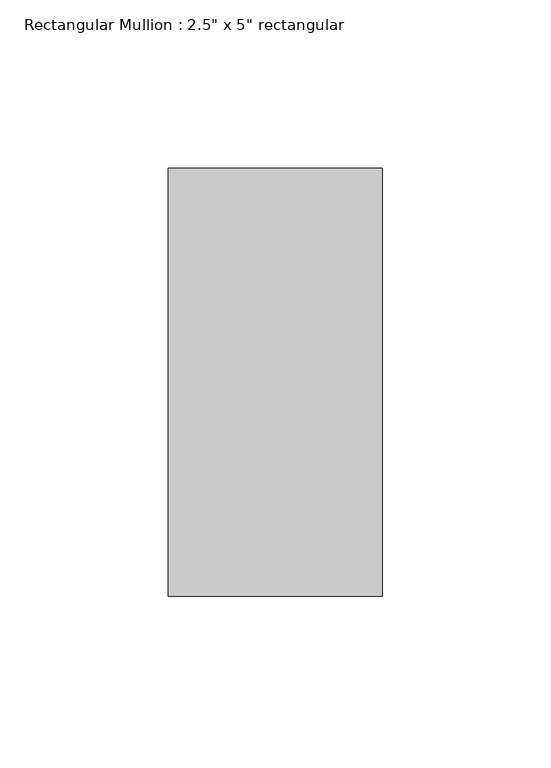
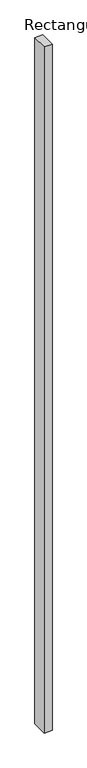
"""IFC4 building model written with IfcOpenShell, lengths in millimetres: member geometry."""

from ifc_helpers import new_model, si_unit, frame, origin, place, context, project, spatial, polyline, outline, extrude, source, transform, mapped, element, save


def member_6e18fad8(model_context):
    return source(origin(), model_context, "Body", "SweptSolid", [
        extrude(outline(polyline([(0.0, 63.5), (0.0, -63.5), (-63.5, -63.5), (-63.5, 63.5), (0.0, 63.5)])), frame((0.0, 0.0, -5793.3288504), z_axis=(0.0, 0.0, 1.0), x_axis=(1.0, 0.0, 0.0)), (0.0, 0.0, 1.0), 5793.3288504),
    ])


if __name__ == "__main__":
    model = new_model("IFC4")
    model_context = context("Model", 3, world=origin())
    ifc_project = project(units=[si_unit("LENGTHUNIT", "METRE", prefix="MILLI")], contexts=[model_context])
    site = spatial("IfcSite", under=ifc_project)
    building = spatial("IfcBuilding", under=site)
    placement = place(None, origin())
    member_shape = member_6e18fad8(model_context)
    element("IfcMember", 1, ObjectType="Rectangular Mullion : 2.5\" x 5\" rectangular", at=placement, inside=building, context=model_context, shape_type="MappedRepresentation", body=[
        mapped(member_shape, transform((0.0, 0.0, 0.0), x_axis=(1.0, 0.0, 0.0), y_axis=(0.0, 1.0, 0.0), z_axis=(0.0, 0.0, 1.0))),
    ])
    save(model, "model.ifc")

# Revit data of these elements
# Type "Rectangular Mullion : 2.5\" x 5\" rectangular"
#   built-in parameter 1007304 = 0.416667 (stored number, unit not read)
#   built-in parameter 1007301 = 0.104167 (stored number, unit not read)
#   built-in parameter 1007300 = 0.104167 (stored number, unit not read)
# Element 1 (IfcMember, "Rectangular Mullion : 2.5\" x 5\" rectangular")
#   Materials on its faces: "Damp-proofing"
# Materials
#   "Damp-proofing": class "Generic", colour RGB 127 127 127, transparency 0, Description = "Damp-proofing", Cost = 0
